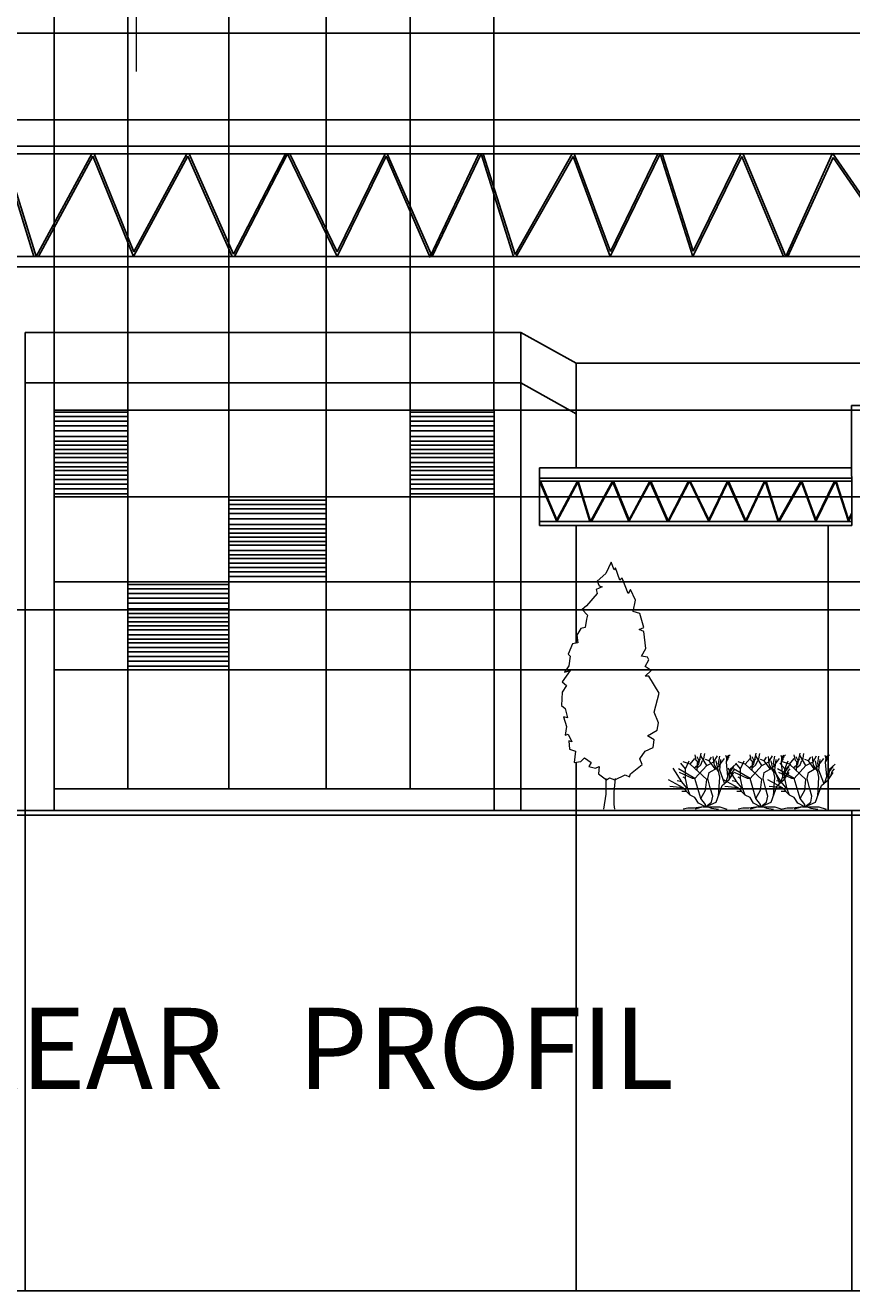
# Model space of a CAD drawing. Units: inches. Extents: x -32109 to 33221, y -19197 to 7608.
# Tile 3 of 25: x -12087 to -6953, y -19197 to -11338. Entities that reach past the tile are written whole.
import ezdxf

# ---------------------------------------------------------------- set-up
doc = ezdxf.new("R2010")
doc.units = ezdxf.units.IN
doc.header["$MEASUREMENT"] = 0
for name, color, linetype, lineweight in [('A-ANNO-DIMS', 2, 'Continuous', 18), ('A-ANNO-NOTE', 2, 'Continuous', 18), ('A-ANNO-TEXT', 7, 'Continuous', 25), ('A-ELEV', 7, 'Continuous', 25), ('L-PLNT', 3, 'Continuous', 13)]:
    doc.layers.add(name, color=color, linetype=linetype, lineweight=lineweight)
doc.styles.get("Standard").update_dxf_attribs({"font": 'arial.ttf'})
doc.dimstyles.get("Standard").update_dxf_attribs({"dimtxt": 0.18, "dimasz": 0.18, "dimexe": 0.18, "dimexo": 0.0625, "dimgap": 0.09, "dimtad": 0, "dimtih": 1, "dimtoh": 1, "dimdec": 4, "dimzin": 0, "dimdsep": 46, "dimtxsty": 'Standard', "dimcen": 0.09, "dimadec": 0, "dimazin": 0, "dimtfac": 1, "dimtdec": 4, "dimtofl": 0, "dimtmove": 0, "dimatfit": 3, "dimfxl": 1, "dimtolj": 1, "dimtzin": 0, "dimarcsym": 0})

# ---------------------------------------------------------------- blocks, each defined once
blk = doc.blocks.new('*U2')
blk.add_lwpolyline([(-2.754, 191.699), (-6.78, 182.851), (-13.682, 176.953), (-11.956, 173.266), (-9.656, 172.529), (-14.257, 170.317), (-13.682, 167.368), (-21.733, 157.783), (-25.184, 154.834), (-21.158, 150.41), (-21.733, 147.461), (-22.884, 140.825), (-26.334, 140.087), (-29.21, 134.926), (-28.635, 129.028), (-32.661, 128.291), (-36.111, 120.18), (-34.386, 118.706), (-35.536, 111.333), (-38.987, 106.171), (-34.386, 107.646), (-40.712, 98.798), (-37.261, 95.849), (-40.712, 90.688), (-41.287, 80.366), (-38.412, 78.154), (-36.686, 70.781), (-39.562, 71.518), (-37.261, 64.145), (-38.412, 57.509), (-36.111, 58.247), (-33.236, 52.348), (-35.536, 53.086), (-34.961, 46.45), (-30.36, 44.975), (-31.51, 36.128), (-26.334, 36.865), (-23.459, 39.814), (-18.283, 36.128), (-20.008, 33.178), (-14.832, 31.704), (-11.956, 33.178), (-12.531, 27.28), (-6.205, 22.856), (-3.905, 24.331), (0.121, 22.856), (8.173, 26.543), (11.624, 25.068), (12.199, 27.28), (21.4, 34.653), (19.675, 39.077), (23.701, 44.975), (30.027, 47.924), (30.602, 53.823), (25.426, 56.772), (32.903, 61.196), (34.053, 67.094), (30.602, 75.205), (34.628, 89.951), (26.576, 103.222), (23.701, 103.222), (28.302, 107.646), (23.701, 110.595), (26.576, 115.756), (25.426, 117.968), (20.825, 118.706), (24.276, 124.604), (22.551, 137.876), (19.1, 139.35), (22.551, 140.825), (19.675, 151.884), (14.499, 153.359), (16.224, 162.207), (12.199, 170.317), (10.473, 167.368), (5.872, 179.165), (4.147, 177.69), (0.696, 187.275), (-0.454, 185.8)], close=True)
for points in [[(-6.813, 23.669), (-6.813, 11.669), (-8.627, 0)], [(0.387, 23.669), (-0.576, 13.271), (-0.576, 3.686), (0, 0)]]:
    blk.add_lwpolyline(points)
blk = doc.blocks.new('*U3')
for p, q in [((-14.88, 18.24), (-12.96, 20.64)), ((-12.471, 19.775), (-12.898, 22.044)), ((-11.28, 19.619), (-12.104, 21.184)), ((-11.433, 18.289), (-10.457, 22.749)), ((-8.16, 17.76), (-10.56, 21.6)), ((-9.48, 19.775), (-8.992, 22.592)), ((-7.2, 19.68), (-6.24, 21.12)), ((-5.086, 17.741), (-5.513, 21.34)), ((-5.28, 19.2), (-3.84, 21.6)), ((-3.84, 16.8), (-0.96, 20.64)), ((-3.377, 18.602), (-2.888, 21.575)), ((-0.508, 21.888), (-0.081, 20.558)), ((-0.203, 19.149), (0.102, 21.34)), ((-0.02, 20.01), (0.896, 21.105)), ((0.041, 20.714), (1.384, 22.044)), ((0.102, 21.34), (0.835, 21.888)), ((-18.24, 11.04), (-21.755, 16.655)), ((-12.96, 12.48), (-19.68, 16.32)), ((-16.8, 16.32), (-18.72, 18.72)), ((-14.88, 18.24), (-17.76, 19.2)), ((-16.8, 16.32), (-15.36, 19.68)), ((-16.8, 12.48), (-16.8, 16.32)), ((-8.16, 12), (-14.88, 18.24)), ((-13.325, 16.724), (-11.433, 18.289)), ((-12.96, 12.48), (-8.16, 17.76)), ((-11.677, 19.071), (-12.471, 19.775)), ((-12.043, 15.628), (-11.921, 18.836)), ((-11.982, 16.802), (-10.579, 18.054)), ((-11.921, 18.836), (-10.64, 20.401)), ((-10.579, 18.054), (-9.846, 19.697)), ((-7.2, 19.68), (-8.64, 20.16)), ((-8.16, 17.76), (-5.28, 19.2)), ((-4.8, 16.32), (-7.2, 19.68)), ((-7.2, 14.88), (-3.84, 16.8)), ((-3.377, 15.315), (-5.086, 17.819)), ((-2.88, 12.96), (-4.32, 19.68)), ((-2.766, 16.802), (-3.377, 18.602)), ((-2.88, 15.84), (-2.4, 20.16)), ((-0.96, 10.56), (-2.88, 15.84)), ((0.346, 13.203), (-0.203, 19.149)), ((-0.142, 19.384), (0.59, 20.401)), ((0.346, 13.203), (1.323, 16.254)), ((1.323, 16.254), (3.642, 18.289)), ((1.44, 15.36), (2.88, 17.28)), ((2.4, 15.36), (3.36, 16.32)), ((-17.76, 8.64), (-23.663, 11.961)), ((-18.24, 11.04), (-20.16, 11.52)), ((-13.92, 12.48), (-19.2, 14.88)), ((-15.84, 8.16), (-18.24, 11.04)), ((-16.8, 12.48), (-17.76, 12.96)), ((-15.84, 8.16), (-16.8, 12.48)), ((-12.96, 12.48), (-13.92, 12.48)), ((-10.56, 4.32), (-12.96, 12.48)), ((-8.64, 7.68), (-8.16, 12)), ((-7.68, 12.48), (-7.2, 14.88)), ((-6.72, 8.64), (-7.68, 12.48)), ((-3.36, 5.28), (-2.88, 12.96)), ((-1.92, 9.6), (0.96, 12)), ((-0.48, 10.8), (0.346, 13.203)), ((0.96, 12), (1.44, 15.36)), ((0.96, 12), (2.88, 14.88)), ((1.92, 13.44), (2.4, 15.36)), ((-17.76, 8.64), (-23.128, 9.222)), ((-16.32, 7.2), (-18.24, 7.2)), ((-14.88, 5.76), (-17.76, 8.64)), ((-14.88, 5.76), (-15.84, 8.16)), ((-12.96, 4.8), (-14.88, 5.76)), ((-10.56, 4.32), (-8.64, 7.68)), ((-5.76, 5.28), (-6.72, 8.64)), ((-6.24, 2.88), (-5.76, 5.28)), ((-4.32, 2.88), (-1.92, 9.6)), ((-15.84, 0.48), (-17.76, 0)), ((-13.44, 0.48), (-15.84, 0.48)), ((-9.6, 0.96), (-13.44, 0.48)), ((-11.52, 2.4), (-12.96, 4.8)), ((-9.6, 0.96), (-12.96, 0)), ((-8.64, 0.96), (-11.52, 2.4)), ((-8.64, 1.92), (-10.56, 4.32)), ((-9.6, 0.96), (-7.68, 0.96)), ((-8.64, 0.96), (-4.32, 2.88)), ((-8.64, 0.96), (-6.24, 2.88)), ((-8.64, 0.96), (-8.64, 1.92)), ((-8.64, 0.96), (-2.88, 0.96)), ((-7.68, 0.96), (-6.24, 0.48)), ((-6.24, 0.48), (-3.36, 0)), ((-2.88, 0.96), (0, 0))]:
    blk.add_line(p, q)
blk = doc.blocks.new('*D13')
at = {"layer": 'A-ANNO-DIMS', "color": 0, "lineweight": -2, "transparency": 16777216}
for p, q in [((-21916.3, -16214.9), (-21916.3, -19197.3)), ((5067.2, -16244.2), (5067.2, -19197.3)), ((-21916.1, -19197.2), (-8425, -19197.2)), ((5067, -19197.2), (-8424.2, -19197.2))]:
    blk.add_line(p, q, dxfattribs=at)
at = {"layer": 'A-ANNO-DIMS', "color": 0, "transparency": 16777216}
for points in [[(-21916.1, -19197.1), (-21916.1, -19197.2), (-21916.3, -19197.2)], [(5067, -19197.1), (5067, -19197.2), (5067.2, -19197.2)]]:
    blk.add_solid(points, dxfattribs=at)
at = {"layer": 'Defpoints', "color": 0, "transparency": 16777216}
for p in [(-21916.3, -16214.8), (5067.2, -16244.1), (5067.2, -19197.2)]:
    blk.add_point(p, dxfattribs=at)
at = {"layer": 'A-ANNO-DIMS', "color": 0, "transparency": 16777216, "insert": (-8424.6, -19197.2), "char_height": 0.18, "attachment_point": 5}
blk.add_mtext('\\A1;26983', dxfattribs=at)
blk = doc.blocks.new('*D14')
at = {"layer": 'A-ANNO-DIMS', "color": 0, "lineweight": -2, "transparency": 16777216}
for p, q in [((-18893.9, -10978.7), (-32108.4, -10978.7)), ((-32108.2, -10978.9), (-32108.2, -13611.2)), ((-32108.2, -16243.9), (-32108.2, -13611.6)), ((5067.1, -16244.1), (-32108.4, -16244.1))]:
    blk.add_line(p, q, dxfattribs=at)
at = {"layer": 'A-ANNO-DIMS', "color": 0, "transparency": 16777216}
for points in [[(-32108.2, -10978.9), (-32108.2, -10978.9), (-32108.2, -10978.7)], [(-32108.2, -16243.9), (-32108.2, -16243.9), (-32108.2, -16244.1)]]:
    blk.add_solid(points, dxfattribs=at)
at = {"layer": 'Defpoints', "color": 0, "transparency": 16777216}
for p in [(-18893.8, -10978.7), (-32108.2, -16244.1), (5067.2, -16244.1)]:
    blk.add_point(p, dxfattribs=at)
at = {"layer": 'A-ANNO-DIMS', "color": 0, "transparency": 16777216, "insert": (-32108.2, -13611.4), "char_height": 0.18, "attachment_point": 5}
blk.add_mtext('\\A1;5265', dxfattribs=at)
blk = doc.blocks.new('*D15')
at = {"layer": 'A-ANNO-DIMS', "color": 0, "lineweight": -2, "transparency": 16777216}
for p, q in [((-8664.1, -16214.9), (-8664.1, -19197.3)), ((-6952.8, -16214.9), (-6952.8, -19197.3)), ((-8664, -19197.2), (-7808.9, -19197.2)), ((-6953, -19197.2), (-7808, -19197.2))]:
    blk.add_line(p, q, dxfattribs=at)
at = {"layer": 'A-ANNO-DIMS', "color": 0, "transparency": 16777216}
for points in [[(-8664, -19197.1), (-8664, -19197.2), (-8664.1, -19197.2)], [(-6953, -19197.1), (-6953, -19197.2), (-6952.8, -19197.2)]]:
    blk.add_solid(points, dxfattribs=at)
at = {"layer": 'Defpoints', "color": 0, "transparency": 16777216}
for p in [(-8664.1, -16214.8), (-6952.8, -16214.8), (-6952.8, -19197.2)]:
    blk.add_point(p, dxfattribs=at)
at = {"layer": 'A-ANNO-DIMS', "color": 0, "transparency": 16777216, "insert": (-7808.5, -19197.2), "char_height": 0.18, "attachment_point": 5}
blk.add_mtext('\\A1;1711.4', dxfattribs=at)
blk = doc.blocks.new('*D23')
at = {"layer": 'A-ANNO-DIMS', "color": 0, "lineweight": -2, "transparency": 16777216}
for p, q in [((-4093.7, -14968.1), (-32108.4, -14968.1)), ((-32108.2, -14968.3), (-32108.2, -15591.3)), ((-32108.2, -16214.6), (-32108.2, -15591.6)), ((-4279, -16214.8), (-32108.4, -16214.8))]:
    blk.add_line(p, q, dxfattribs=at)
at = {"layer": 'A-ANNO-DIMS', "color": 0, "transparency": 16777216}
for points in [[(-32108.2, -14968.3), (-32108.2, -14968.3), (-32108.2, -14968.1)], [(-32108.2, -16214.6), (-32108.2, -16214.6), (-32108.2, -16214.8)]]:
    blk.add_solid(points, dxfattribs=at)
at = {"layer": 'Defpoints', "color": 0, "transparency": 16777216}
for p in [(-32108.2, -14968.1), (-4093.7, -14968.1), (-4279, -16214.8)]:
    blk.add_point(p, dxfattribs=at)
at = {"layer": 'A-ANNO-DIMS', "color": 0, "transparency": 16777216, "insert": (-32108.2, -15591.4), "char_height": 0.18, "attachment_point": 5}
blk.add_mtext('\\A1;1246.7', dxfattribs=at)
blk = doc.blocks.new('*D83')
at = {"layer": 'A-ANNO-DIMS', "color": 0, "lineweight": -2, "transparency": 16777216}
for p, q in [((-12087.2, -16214.9), (-12087.2, -19197.3)), ((-8664.1, -16214.9), (-8664.1, -19197.3)), ((-12087, -19197.2), (-10376, -19197.2)), ((-8664.3, -19197.2), (-10375.3, -19197.2))]:
    blk.add_line(p, q, dxfattribs=at)
at = {"layer": 'A-ANNO-DIMS', "color": 0, "transparency": 16777216}
for points in [[(-12087, -19197.1), (-12087, -19197.2), (-12087.2, -19197.2)], [(-8664.3, -19197.1), (-8664.3, -19197.2), (-8664.1, -19197.2)]]:
    blk.add_solid(points, dxfattribs=at)
at = {"layer": 'Defpoints', "color": 0, "transparency": 16777216}
for p in [(-12087.2, -16214.8), (-8664.1, -16214.8), (-8664.1, -19197.2)]:
    blk.add_point(p, dxfattribs=at)
at = {"layer": 'A-ANNO-DIMS', "color": 0, "transparency": 16777216, "insert": (-10375.7, -19197.2), "char_height": 0.18, "attachment_point": 5}
blk.add_mtext('\\A1;3423', dxfattribs=at)
blk = doc.blocks.new('*D88')
at = {"layer": 'A-ANNO-DIMS', "color": 0, "lineweight": -2, "transparency": 16777216}
for p, q in [((-6450, -11924), (-32108.4, -11924)), ((-32108.2, -11924.1), (-32108.2, -12380.7)), ((-32108.2, -12837.6), (-32108.2, -12381)), ((-6450, -12837.7), (-32108.4, -12837.7))]:
    blk.add_line(p, q, dxfattribs=at)
at = {"layer": 'A-ANNO-DIMS', "color": 0, "transparency": 16777216}
for points in [[(-32108.2, -11924.1), (-32108.2, -11924.1), (-32108.2, -11924)], [(-32108.2, -12837.6), (-32108.2, -12837.6), (-32108.2, -12837.7)]]:
    blk.add_solid(points, dxfattribs=at)
at = {"layer": 'Defpoints', "color": 0, "transparency": 16777216}
for p in [(-6450, -11924), (-32108.2, -12837.7), (-6450, -12837.7)]:
    blk.add_point(p, dxfattribs=at)
at = {"layer": 'A-ANNO-DIMS', "color": 0, "transparency": 16777216, "insert": (-32108.2, -12380.9), "char_height": 0.18, "attachment_point": 5}
blk.add_mtext('\\A1;913.8', dxfattribs=at)
blk = doc.blocks.new('*D92')
at = {"layer": 'A-ANNO-DIMS', "color": 0, "lineweight": -2, "transparency": 16777216}
for p, q in [((-8664.1, -13437.2), (9252.7, -13437.2)), ((9252.5, -13437.4), (9252.5, -14825.8)), ((9252.5, -16214.6), (9252.5, -14826.2)), ((-8664.1, -16214.8), (9252.7, -16214.8))]:
    blk.add_line(p, q, dxfattribs=at)
at = {"layer": 'A-ANNO-DIMS', "color": 0, "transparency": 16777216}
for points in [[(9252.5, -13437.4), (9252.5, -13437.4), (9252.5, -13437.2)], [(9252.5, -16214.6), (9252.5, -16214.6), (9252.5, -16214.8)]]:
    blk.add_solid(points, dxfattribs=at)
at = {"layer": 'Defpoints', "color": 0, "transparency": 16777216}
for p in [(-8664.1, -13437.2), (-8664.1, -16214.8), (9252.5, -16214.8)]:
    blk.add_point(p, dxfattribs=at)
at = {"layer": 'A-ANNO-DIMS', "color": 0, "transparency": 16777216, "insert": (9252.5, -14826), "char_height": 0.18, "attachment_point": 5}
blk.add_mtext('\\A1;2777.6', dxfattribs=at)
blk = doc.blocks.new('*D94')
at = {"layer": 'A-ANNO-DIMS', "color": 0, "lineweight": -2, "transparency": 16777216}
for p, q in [((-11907.7, -13729), (-11907.7, -7335)), ((-11907.5, -7335.2), (-11679.5, -7335.2)), ((-11450.7, -7335.2), (-11678.7, -7335.2)), ((-11450.5, -13729), (-11450.5, -7335))]:
    blk.add_line(p, q, dxfattribs=at)
at = {"layer": 'A-ANNO-DIMS', "color": 0, "transparency": 16777216}
for points in [[(-11907.5, -7335.1), (-11907.5, -7335.2), (-11907.7, -7335.2)], [(-11450.7, -7335.1), (-11450.7, -7335.2), (-11450.5, -7335.2)]]:
    blk.add_solid(points, dxfattribs=at)
at = {"layer": 'Defpoints', "color": 0, "transparency": 16777216}
for p in [(-11450.5, -7335.2), (-11907.7, -13729), (-11450.5, -13729)]:
    blk.add_point(p, dxfattribs=at)
at = {"layer": 'A-ANNO-DIMS', "color": 0, "transparency": 16777216, "insert": (-11679.1, -7335.2), "char_height": 0.18, "attachment_point": 5}
blk.add_mtext('\\A1;457.2', dxfattribs=at)
blk = doc.blocks.new('*D95')
at = {"layer": 'A-ANNO-DIMS', "color": 0, "lineweight": -2, "transparency": 16777216}
for p, q in [((-11450.5, -13729), (-11450.5, -7335)), ((-11450.3, -7335.2), (-11137.2, -7335.2)), ((-10823.3, -7335.2), (-11136.4, -7335.2)), ((-10823.2, -13729), (-10823.2, -7335))]:
    blk.add_line(p, q, dxfattribs=at)
at = {"layer": 'A-ANNO-DIMS', "color": 0, "transparency": 16777216}
for points in [[(-11450.3, -7335.1), (-11450.3, -7335.2), (-11450.5, -7335.2)], [(-10823.3, -7335.1), (-10823.3, -7335.2), (-10823.2, -7335.2)]]:
    blk.add_solid(points, dxfattribs=at)
at = {"layer": 'Defpoints', "color": 0, "transparency": 16777216}
for p in [(-10823.2, -7335.2), (-11450.5, -13729), (-10823.2, -13729)]:
    blk.add_point(p, dxfattribs=at)
at = {"layer": 'A-ANNO-DIMS', "color": 0, "transparency": 16777216, "insert": (-11136.8, -7335.2), "char_height": 0.18, "attachment_point": 5}
blk.add_mtext('\\A1;627.3', dxfattribs=at)
blk = doc.blocks.new('*D96')
at = {"layer": 'A-ANNO-DIMS', "color": 0, "lineweight": -2, "transparency": 16777216}
for p, q in [((-10823.2, -13729), (-10823.2, -7335)), ((-10823, -7335.2), (-10520.4, -7335.2)), ((-10217.3, -7335.2), (-10519.9, -7335.2)), ((-10217.1, -13729), (-10217.1, -7335))]:
    blk.add_line(p, q, dxfattribs=at)
at = {"layer": 'A-ANNO-DIMS', "color": 0, "transparency": 16777216}
for points in [[(-10823, -7335.1), (-10823, -7335.2), (-10823.2, -7335.2)], [(-10217.3, -7335.1), (-10217.3, -7335.2), (-10217.1, -7335.2)]]:
    blk.add_solid(points, dxfattribs=at)
at = {"layer": 'Defpoints', "color": 0, "transparency": 16777216}
for p in [(-10217.1, -7335.2), (-10823.2, -13729), (-10217.1, -13729)]:
    blk.add_point(p, dxfattribs=at)
at = {"layer": 'A-ANNO-DIMS', "color": 0, "transparency": 16777216, "insert": (-10520.1, -7335.2), "char_height": 0.18, "attachment_point": 5}
blk.add_mtext('\\A1;606', dxfattribs=at)
blk = doc.blocks.new('*D97')
at = {"layer": 'A-ANNO-DIMS', "color": 0, "lineweight": -2, "transparency": 16777216}
for p, q in [((-10217.1, -13729), (-10217.1, -7335)), ((-10216.9, -7335.2), (-9956.9, -7335.2)), ((-9696.3, -7335.2), (-9956.4, -7335.2)), ((-9696.1, -13729), (-9696.1, -7335))]:
    blk.add_line(p, q, dxfattribs=at)
at = {"layer": 'A-ANNO-DIMS', "color": 0, "transparency": 16777216}
for points in [[(-10216.9, -7335.1), (-10216.9, -7335.2), (-10217.1, -7335.2)], [(-9696.3, -7335.1), (-9696.3, -7335.2), (-9696.1, -7335.2)]]:
    blk.add_solid(points, dxfattribs=at)
at = {"layer": 'Defpoints', "color": 0, "transparency": 16777216}
for p in [(-9696.1, -7335.2), (-10217.1, -13729), (-9696.1, -13729)]:
    blk.add_point(p, dxfattribs=at)
at = {"layer": 'A-ANNO-DIMS', "color": 0, "transparency": 16777216, "insert": (-9956.6, -7335.2), "char_height": 0.18, "attachment_point": 5}
blk.add_mtext('\\A1;521', dxfattribs=at)
blk = doc.blocks.new('*D98')
at = {"layer": 'A-ANNO-DIMS', "color": 0, "lineweight": -2, "transparency": 16777216}
for p, q in [((-9696.1, -13729), (-9696.1, -7335)), ((-9696, -7335.2), (-9435.9, -7335.2)), ((-9175.3, -7335.2), (-9435.4, -7335.2)), ((-9175.2, -13729), (-9175.2, -7335))]:
    blk.add_line(p, q, dxfattribs=at)
at = {"layer": 'A-ANNO-DIMS', "color": 0, "transparency": 16777216}
for points in [[(-9696, -7335.1), (-9696, -7335.2), (-9696.1, -7335.2)], [(-9175.3, -7335.1), (-9175.3, -7335.2), (-9175.2, -7335.2)]]:
    blk.add_solid(points, dxfattribs=at)
at = {"layer": 'Defpoints', "color": 0, "transparency": 16777216}
for p in [(-9175.2, -7335.2), (-9696.1, -13729), (-9175.2, -13729)]:
    blk.add_point(p, dxfattribs=at)
at = {"layer": 'A-ANNO-DIMS', "color": 0, "transparency": 16777216, "insert": (-9435.6, -7335.2), "char_height": 0.18, "attachment_point": 5}
blk.add_mtext('\\A1;521', dxfattribs=at)
blk = doc.blocks.new('*D99')
at = {"layer": 'A-ANNO-DIMS', "color": 0, "lineweight": -2, "transparency": 16777216}
for p, q in [((-9175.1, -13729), (9252.7, -13729)), ((9252.5, -13729.2), (9252.5, -13997.5)), ((9252.5, -14266.2), (9252.5, -13997.9)), ((-9175.1, -14266.4), (9252.7, -14266.4))]:
    blk.add_line(p, q, dxfattribs=at)
at = {"layer": 'A-ANNO-DIMS', "color": 0, "transparency": 16777216}
for points in [[(9252.5, -13729.2), (9252.5, -13729.2), (9252.5, -13729)], [(9252.5, -14266.2), (9252.5, -14266.2), (9252.5, -14266.4)]]:
    blk.add_solid(points, dxfattribs=at)
at = {"layer": 'Defpoints', "color": 0, "transparency": 16777216}
for p in [(-9175.2, -13729), (-9175.2, -14266.4), (9252.5, -14266.4)]:
    blk.add_point(p, dxfattribs=at)
at = {"layer": 'A-ANNO-DIMS', "color": 0, "transparency": 16777216, "insert": (9252.5, -13997.7), "char_height": 0.18, "attachment_point": 5}
blk.add_mtext('\\A1;537.4', dxfattribs=at)
blk = doc.blocks.new('*D100')
at = {"layer": 'A-ANNO-DIMS', "color": 0, "lineweight": -2, "transparency": 16777216}
for p, q in [((-9175.1, -14266.4), (9252.7, -14266.4)), ((9252.5, -14266.6), (9252.5, -14530.6)), ((9252.5, -14794.9), (9252.5, -14530.9)), ((-9175.1, -14795.1), (9252.7, -14795.1))]:
    blk.add_line(p, q, dxfattribs=at)
at = {"layer": 'A-ANNO-DIMS', "color": 0, "transparency": 16777216}
for points in [[(9252.5, -14266.6), (9252.5, -14266.6), (9252.5, -14266.4)], [(9252.5, -14794.9), (9252.5, -14794.9), (9252.5, -14795.1)]]:
    blk.add_solid(points, dxfattribs=at)
at = {"layer": 'Defpoints', "color": 0, "transparency": 16777216}
for p in [(-9175.2, -14266.4), (-9175.2, -14795.1), (9252.5, -14795.1)]:
    blk.add_point(p, dxfattribs=at)
at = {"layer": 'A-ANNO-DIMS', "color": 0, "transparency": 16777216, "insert": (9252.5, -14530.7), "char_height": 0.18, "attachment_point": 5}
blk.add_mtext('\\A1;528.7', dxfattribs=at)
blk = doc.blocks.new('*D101')
at = {"layer": 'A-ANNO-DIMS', "color": 0, "lineweight": -2, "transparency": 16777216}
for p, q in [((-9175.1, -14795.1), (9252.7, -14795.1)), ((9252.5, -14795.3), (9252.5, -15068.4)), ((9252.5, -15341.8), (9252.5, -15068.7)), ((-9175.1, -15342), (9252.7, -15342))]:
    blk.add_line(p, q, dxfattribs=at)
at = {"layer": 'A-ANNO-DIMS', "color": 0, "transparency": 16777216}
for points in [[(9252.5, -14795.3), (9252.5, -14795.3), (9252.5, -14795.1)], [(9252.5, -15341.8), (9252.5, -15341.8), (9252.5, -15342)]]:
    blk.add_solid(points, dxfattribs=at)
at = {"layer": 'Defpoints', "color": 0, "transparency": 16777216}
for p in [(-9175.2, -14795.1), (-9175.2, -15342), (9252.5, -15342)]:
    blk.add_point(p, dxfattribs=at)
at = {"layer": 'A-ANNO-DIMS', "color": 0, "transparency": 16777216, "insert": (9252.5, -15068.6), "char_height": 0.18, "attachment_point": 5}
blk.add_mtext('\\A1;546.9', dxfattribs=at)
blk = doc.blocks.new('*D102')
at = {"layer": 'A-ANNO-DIMS', "color": 0, "lineweight": -2, "transparency": 16777216}
for p, q in [((-9175.1, -15342), (9252.7, -15342)), ((9252.5, -15342.2), (9252.5, -15710.5)), ((9252.5, -16079.1), (9252.5, -15710.8)), ((-9175.1, -16079.3), (9252.7, -16079.3))]:
    blk.add_line(p, q, dxfattribs=at)
at = {"layer": 'A-ANNO-DIMS', "color": 0, "transparency": 16777216}
for points in [[(9252.5, -15342.2), (9252.5, -15342.2), (9252.5, -15342)], [(9252.5, -16079.1), (9252.5, -16079.1), (9252.5, -16079.3)]]:
    blk.add_solid(points, dxfattribs=at)
at = {"layer": 'Defpoints', "color": 0, "transparency": 16777216}
for p in [(-9175.2, -15342), (-9175.2, -16079.3), (9252.5, -16079.3)]:
    blk.add_point(p, dxfattribs=at)
at = {"layer": 'A-ANNO-DIMS', "color": 0, "transparency": 16777216, "insert": (9252.5, -15710.6), "char_height": 0.18, "attachment_point": 5}
blk.add_mtext('\\A1;737.3', dxfattribs=at)
blk = doc.blocks.new('*D111')
at = {"layer": 'A-ANNO-DIMS', "color": 0, "lineweight": -2, "transparency": 16777216}
for p, q in [((-6954.6, -13699.5), (9252.7, -13699.5)), ((9252.5, -13699.6), (9252.5, -14957)), ((9252.5, -16214.6), (9252.5, -14957.3)), ((-6952.7, -16214.8), (9252.7, -16214.8))]:
    blk.add_line(p, q, dxfattribs=at)
at = {"layer": 'A-ANNO-DIMS', "color": 0, "transparency": 16777216}
for points in [[(9252.5, -13699.6), (9252.5, -13699.6), (9252.5, -13699.5)], [(9252.5, -16214.6), (9252.5, -16214.6), (9252.5, -16214.8)]]:
    blk.add_solid(points, dxfattribs=at)
at = {"layer": 'Defpoints', "color": 0, "transparency": 16777216}
for p in [(-6954.6, -13699.5), (-6952.8, -16214.8), (9252.5, -16214.8)]:
    blk.add_point(p, dxfattribs=at)
at = {"layer": 'A-ANNO-DIMS', "color": 0, "transparency": 16777216, "insert": (9252.5, -14957.1), "char_height": 0.18, "attachment_point": 5}
blk.add_mtext('\\A1;2515.4', dxfattribs=at)
blk = doc.blocks.new('*D159')
at = {"layer": 'A-ANNO-DIMS', "color": 0, "lineweight": -2, "transparency": 16777216}
for p, q in [((-6094.7, -11386.3), (-32108.4, -11386.3)), ((-32108.2, -11386.4), (-32108.2, -13800.4)), ((-32108.2, -16214.6), (-32108.2, -13800.7)), ((-6952.8, -16214.8), (-32108.4, -16214.8))]:
    blk.add_line(p, q, dxfattribs=at)
at = {"layer": 'A-ANNO-DIMS', "color": 0, "transparency": 16777216}
for points in [[(-32108.2, -11386.4), (-32108.2, -11386.4), (-32108.2, -11386.3)], [(-32108.2, -16214.6), (-32108.2, -16214.6), (-32108.2, -16214.8)]]:
    blk.add_solid(points, dxfattribs=at)
at = {"layer": 'Defpoints', "color": 0, "transparency": 16777216}
for p in [(-6094.7, -11386.3), (-32108.2, -16214.8), (-6952.8, -16214.8)]:
    blk.add_point(p, dxfattribs=at)
at = {"layer": 'A-ANNO-DIMS', "color": 0, "transparency": 16777216, "insert": (-32108.2, -13800.5), "char_height": 0.18, "attachment_point": 5}
blk.add_mtext('\\A1;4828.6', dxfattribs=at)

msp = doc.modelspace()

# ---------------------------------------------------------------- linework, layer by layer
at = {"layer": 'A-ANNO-NOTE'}
msp.add_line((-11395.932, -11625.267), (-11395.932, -9225.16), dxfattribs=at)
at = {"layer": 'A-ELEV'}
for p, q in [((-6449.955, -11923.964), (-13434.383, -11923.964)), ((-13434.383, -12088.725), (-6449.955, -12088.725)), ((-6449.955, -12135.164), (-13434.383, -12135.164)), ((-12033.808, -12773.917), (-12224.259, -12151.939)), ((-12020.326, -12774.298), (-12215.76, -12136.047)), ((-11673.548, -12136.139), (-12020.326, -12774.298)), ((-11667.326, -12151.455), (-12005.574, -12773.917)), ((-11414.231, -12774.408), (-11667.326, -12151.455)), ((-11412.588, -12744.499), (-11660.15, -12135.164)), ((-11076.952, -12150.578), (-11414.231, -12774.408)), ((-11083.147, -12135.164), (-11412.588, -12744.499)), ((-10802.158, -12773.917), (-11076.952, -12150.578)), ((-10794.601, -12759.378), (-11069.259, -12136.348)), ((-10471.397, -12135.164), (-10794.601, -12759.378)), ((-10457.568, -12136.249), (-10787.983, -12774.39)), ((-10148.844, -12774.323), (-10457.568, -12136.249)), ((-10148.814, -12745.042), (-10443.896, -12135.164)), ((-9845.785, -12151.2), (-10148.844, -12774.323)), ((-9852.197, -12135.164), (-10148.814, -12745.042)), ((-9570.82, -12779.373), (-9845.785, -12151.2)), ((-9559.112, -12774.249), (-9838.443, -12136.104)), ((-9269.526, -12135.164), (-9570.655, -12768.763)), ((-9255.782, -12136.019), (-9559.112, -12774.249)), ((-9053.761, -12773.917), (-9255.782, -12136.019)), ((-9044.471, -12760.923), (-9242.647, -12135.164)), ((-8690.019, -12136.482), (-9044.471, -12760.923)), ((-8684.219, -12152.151), (-9037.152, -12773.917)), ((-8453.963, -12774.128), (-8684.219, -12152.151)), ((-8452.368, -12741.626), (-8676.88, -12135.164)), ((-8143.814, -12136.351), (-8453.963, -12774.128)), ((-8157.448, -12135.164), (-8452.368, -12741.626)), ((-7939.481, -12774.128), (-8143.814, -12136.351)), ((-7936.987, -12740.027), (-8130.775, -12135.164)), ((-7634.998, -12153.442), (-7939.481, -12774.128)), ((-7638.981, -12132.545), (-7936.987, -12740.027)), ((-7376.899, -12773.917), (-7634.998, -12153.442)), ((-7362.969, -12774.128), (-7627.508, -12138.174)), ((-7071.065, -12132.707), (-7362.969, -12774.128)), ((-7068.778, -12158.535), (-7348.832, -12773.917)), ((-6628.917, -12773.917), (-7071.065, -12132.707)), ((-6644.441, -12773.917), (-7068.778, -12158.535)), ((-13434.383, -12773.917), (-6449.955, -12773.917)), ((-10787.983, -12774.39), (-10788.191, -12773.917)), ((-6449.955, -12837.747), (-13434.383, -12837.747)), ((-12087.226, -12837.489), (-9386.71, -12837.747)), ((-9070.682, -12837.747), (-11681.584, -12837.747)), ((-12087.226, -13436.327), (-12087.226, -13244.79)), ((-12087.226, -13244.79), (-9009.085, -13244.79)), ((-9009.085, -13244.79), (-8664.143, -13437.203)), ((-9009.085, -13244.79), (-9009.085, -13557.609)), ((-12087.226, -14445.256), (-12087.226, -13436.327)), ((-8664.143, -13750.022), (-8664.143, -13437.203)), ((-9009.085, -13557.609), (-12087.226, -13557.609)), ((-9009.085, -13557.609), (-9009.085, -14445.256)), ((-9009.085, -13557.609), (-8664.143, -13750.022)), ((-11907.664, -16214.811), (-11907.664, -13729.028)), ((-11907.664, -13729.028), (-9175.157, -13729.028)), ((-11907.664, -13741.003), (-11450.474, -13741.003)), ((-11450.474, -16079.3), (-11450.474, -13729.028)), ((-10823.167, -16079.3), (-10823.167, -13729.028)), ((-10217.124, -16079.3), (-10217.124, -13729.028)), ((-9699.007, -13741.003), (-9175.157, -13741.003)), ((-9696.14, -16079.3), (-9696.14, -13729.028)), ((-9175.157, -13729.028), (-9175.157, -16214.811)), ((-8664.143, -14086.672), (-8664.143, -13750.022)), ((-6954.623, -13834.091), (-6954.623, -13699.459)), ((-6954.623, -13699.459), (-6943.296, -13699.459)), ((-11907.664, -13768.233), (-11450.474, -13768.233)), ((-11907.664, -13796.415), (-11450.474, -13796.415)), ((-11907.664, -13824.813), (-11450.474, -13824.813)), ((-9699.007, -13768.233), (-9175.157, -13768.233)), ((-9699.007, -13796.415), (-9175.157, -13796.415)), ((-9699.007, -13824.813), (-9175.157, -13824.813)), ((-11907.664, -13857.368), (-11450.474, -13857.368)), ((-11907.664, -13892), (-11450.474, -13892)), ((-9699.007, -13857.368), (-9175.157, -13857.368)), ((-9699.007, -13892), (-9175.157, -13892)), ((-6954.623, -13834.091), (-6952.774, -14445.256)), ((-11907.664, -13919.943), (-11450.474, -13919.943)), ((-11907.664, -13946.263), (-11450.474, -13946.263)), ((-11907.664, -13971.892), (-11450.474, -13971.892)), ((-9699.007, -13919.943), (-9175.157, -13919.943)), ((-9699.007, -13946.263), (-9175.157, -13946.263)), ((-9699.007, -13971.892), (-9175.157, -13971.892)), ((-11907.664, -13997.52), (-11450.474, -13997.52)), ((-11907.664, -14021.762), (-11450.474, -14021.762)), ((-11907.664, -14053.653), (-11450.474, -14053.653)), ((-9699.007, -13997.52), (-9175.157, -13997.52)), ((-9699.007, -14021.762), (-9175.157, -14021.762)), ((-9699.007, -14053.653), (-9175.157, -14053.653)), ((-11907.664, -14080.587), (-11450.474, -14080.587)), ((-11907.664, -14103.611), (-11450.474, -14103.611)), ((-11907.664, -14132.215), (-11450.474, -14132.215)), ((-9699.007, -14080.587), (-9175.157, -14080.587)), ((-9699.007, -14103.611), (-9175.157, -14103.611)), ((-9699.007, -14132.215), (-9175.157, -14132.215)), ((-6953.859, -14086.672), (-8891.72, -14086.672)), ((-8891.72, -14086.672), (-8891.72, -14151.327)), ((-11907.664, -14159.446), (-11450.474, -14159.446)), ((-11907.664, -14187.627), (-11450.474, -14187.627)), ((-11907.664, -14216.026), (-11450.474, -14216.026)), ((-9699.007, -14159.446), (-9175.157, -14159.446)), ((-9699.007, -14187.627), (-9175.157, -14187.627)), ((-9699.007, -14216.026), (-9175.157, -14216.026)), ((-8891.72, -14151.327), (-6953.663, -14151.327)), ((-8891.72, -14169.551), (-8891.72, -14151.327)), ((-8785.46, -14420.382), (-8891.72, -14169.464)), ((-6953.608, -14169.551), (-8891.72, -14169.551)), ((-8891.72, -14169.551), (-8891.72, -14420.208)), ((-8784.934, -14408.765), (-8886.237, -14169.551)), ((-8654.831, -14176.133), (-8785.46, -14420.382)), ((-8656.997, -14169.551), (-8784.934, -14408.765)), ((-8580.094, -14420.208), (-8654.831, -14176.133)), ((-8574.804, -14420.357), (-8651.495, -14169.897)), ((-8438.722, -14169.933), (-8574.804, -14420.357)), ((-8436.281, -14175.943), (-8569.015, -14420.208)), ((-8336.962, -14420.4), (-8436.281, -14175.943)), ((-8336.317, -14408.664), (-8433.465, -14169.551)), ((-8204.608, -14175.599), (-8336.962, -14420.4)), ((-8207.039, -14169.551), (-8336.317, -14408.664)), ((-8096.774, -14420.208), (-8204.608, -14175.599)), ((-8093.809, -14414.502), (-8201.589, -14170.015)), ((-7966.978, -14169.551), (-8093.809, -14414.502)), ((-7961.551, -14169.976), (-8091.212, -14420.394)), ((-7840.403, -14420.367), (-7961.551, -14169.976)), ((-7840.391, -14408.877), (-7956.186, -14169.551)), ((-7721.477, -14175.843), (-7840.403, -14420.367)), ((-7723.994, -14169.551), (-7840.391, -14408.877)), ((-7613.576, -14422.349), (-7721.477, -14175.843)), ((-7608.982, -14420.338), (-7718.596, -14169.919)), ((-7495.344, -14169.551), (-7613.512, -14418.185)), ((-7489.95, -14169.886), (-7608.982, -14420.338)), ((-7410.674, -14420.208), (-7489.95, -14169.886)), ((-7407.029, -14415.109), (-7484.796, -14169.551)), ((-7267.936, -14170.068), (-7407.029, -14415.109)), ((-7265.659, -14176.217), (-7404.156, -14420.208)), ((-7175.303, -14420.291), (-7265.659, -14176.217)), ((-7174.677, -14407.536), (-7262.78, -14169.551)), ((-7053.596, -14170.016), (-7175.303, -14420.291)), ((-7058.946, -14169.551), (-7174.677, -14407.536)), ((-6973.412, -14420.291), (-7053.596, -14170.016)), ((-6972.433, -14406.909), (-7048.479, -14169.551)), ((-11907.664, -14248.581), (-11450.474, -14248.581)), ((-11907.664, -14266.38), (-9175.157, -14266.38)), ((-10823.167, -14286.356), (-10217.124, -14286.356)), ((-9699.007, -14248.581), (-9175.157, -14248.581)), ((-10823.167, -14313.587), (-10217.124, -14313.587)), ((-10823.167, -14341.768), (-10217.124, -14341.768)), ((-10823.167, -14370.167), (-10217.124, -14370.167)), ((-6952.975, -14378.631), (-6973.412, -14420.291)), ((-6953.01, -14367.314), (-6972.433, -14406.909)), ((-12087.226, -14445.256), (-12087.226, -16214.811)), ((-10823.167, -14402.721), (-10217.124, -14402.721)), ((-10823.167, -14437.354), (-10217.124, -14437.354)), ((-9009.085, -14445.256), (-9009.085, -16214.811)), ((-8891.72, -14420.208), (-6952.85, -14420.208)), ((-8891.72, -14445.256), (-8891.72, -14420.208)), ((-6952.774, -14445.256), (-8891.72, -14445.256)), ((-8664.143, -14445.256), (-8664.143, -15175.201)), ((-8091.212, -14420.394), (-8091.294, -14420.208)), ((-7098.526, -14445.256), (-7098.526, -16214.811)), ((-10823.167, -14465.296), (-10217.124, -14465.296)), ((-10823.167, -14491.617), (-10217.124, -14491.617)), ((-10823.167, -14517.245), (-10217.124, -14517.245)), ((-10823.167, -14542.873), (-10217.124, -14542.873)), ((-10823.167, -14567.116), (-10217.124, -14567.116)), ((-10823.167, -14599.007), (-10217.124, -14599.007)), ((-10823.167, -14625.941), (-10217.124, -14625.941)), ((-10823.167, -14648.965), (-10217.124, -14648.965)), ((-10823.167, -14677.569), (-10217.124, -14677.569)), ((-10823.167, -14704.8), (-10217.124, -14704.8)), ((-10823.167, -14732.981), (-10217.124, -14732.981)), ((-10823.167, -14761.38), (-10217.124, -14761.38)), ((-11907.664, -14795.117), (-9175.157, -14795.117)), ((-11450.474, -14811.581), (-10823.167, -14811.581)), ((-11450.474, -14838.812), (-10823.167, -14838.812)), ((-11450.474, -14866.993), (-10823.167, -14866.993)), ((-11450.474, -14895.392), (-10823.167, -14895.392)), ((-11450.474, -14927.946), (-10823.167, -14927.946)), ((-11450.474, -14962.579), (-10823.167, -14962.579)), ((-11450.474, -14990.521), (-10823.167, -14990.521)), ((-11450.474, -15016.842), (-10823.167, -15016.842)), ((-11450.474, -15042.47), (-10823.167, -15042.47)), ((-11450.474, -15068.098), (-10823.167, -15068.098)), ((-11450.474, -15092.341), (-10823.167, -15092.341)), ((-11450.474, -15124.232), (-10823.167, -15124.232)), ((-11450.474, -15151.166), (-10823.167, -15151.166)), ((-11450.474, -15174.19), (-10823.167, -15174.19)), ((-11450.474, -15202.794), (-10823.167, -15202.794)), ((-11450.474, -15230.025), (-10823.167, -15230.025)), ((-11450.474, -15258.206), (-10823.167, -15258.206)), ((-11450.474, -15286.605), (-10823.167, -15286.605)), ((-11450.474, -15319.159), (-10823.167, -15319.159)), ((-11907.664, -15341.992), (-9175.157, -15341.992)), ((-8664.143, -15915.078), (-8664.143, -16214.811)), ((-11907.664, -16079.3), (-9175.157, -16079.3)), ((-12087.226, -16214.811), (7362.494, -16214.811)), ((-1417.009, -16214.811), (-10157.643, -16214.811))]:
    msp.add_line(p, q, dxfattribs=at)

# ---------------------------------------------------------------- block references
at = {"layer": 'L-PLNT'}
for name, p, xscale, yscale, zscale in [('*U2', (-8425.752, -16206.195), 8.003528136912784, 8.003528136912784, 8.003528136912784), ('*U3', (-7728.374, -16206.683), 15.30854395898754, 15.30854395898754, 15.30854395898754), ('*U3', (-7386.265, -16206.683), 15.30854395898754, 15.30854395898754, 15.30854395898754), ('*U3', (-7111.901, -16206.683), 15.30854395898754, 15.30854395898754, 15.30854395898754)]:
    msp.add_blockref(name, p, dxfattribs=dict(at, xscale=xscale, yscale=yscale, zscale=zscale))

# ---------------------------------------------------------------- texts
at = {"layer": 'A-ANNO-TEXT'}
msp.add_text('SERVICE   AND   MECHNICAL  SPINE   REAR   PROFIL  ', height=504.21831, dxfattribs=at).set_placement((-24112.83, -17944.243))

# ---------------------------------------------------------------- dimensions: what is measured, and where the dimension line sits
at = {"layer": 'A-ANNO-DIMS'}
for base, p1, p2, override, picture, middle in [((-11450.474, -7335.16), (-11907.664, -13729.028), (-11450.474, -13729.028), {"dimdec": 1, "dimlfac": 1, "dimrnd": 0, "dimzin": 0, "dimdsep": 46, "dimlunit": 2}, '*D94', (-11679.069, -7335.16)), ((-10823.167, -7335.16), (-11450.474, -13729.028), (-10823.167, -13729.028), {"dimdec": 1, "dimlfac": 1, "dimrnd": 0, "dimzin": 0, "dimdsep": 46, "dimlunit": 2}, '*D95', (-11136.82, -7335.16)), ((-10217.124, -7335.16), (-10823.167, -13729.028), (-10217.124, -13729.028), {"dimdec": 0, "dimlfac": 1, "dimrnd": 0, "dimzin": 0, "dimdsep": 46, "dimlunit": 2}, '*D96', (-10520.145, -7335.16)), ((-9696.14, -7335.16), (-10217.124, -13729.028), (-9696.14, -13729.028), {"dimdec": 0, "dimlfac": 1, "dimrnd": 0, "dimzin": 0, "dimdsep": 46, "dimlunit": 2}, '*D97', (-9956.632, -7335.16)), ((-9175.157, -7335.16), (-9696.14, -13729.028), (-9175.157, -13729.028), {"dimdec": 0, "dimlfac": 1, "dimrnd": 0, "dimzin": 0, "dimdsep": 46, "dimlunit": 2}, '*D98', (-9435.648, -7335.16)), ((5067.151, -19197.169), (-21916.328, -16214.811), (5067.151, -16244.113), {"dimdec": 0, "dimlfac": 1, "dimrnd": 0, "dimzin": 0, "dimdsep": 46, "dimlunit": 2}, '*D13', (-8424.588, -19197.169)), ((-8664.143, -19197.169), (-12087.226, -16214.811), (-8664.143, -16214.811), {"dimdec": 0, "dimlfac": 1, "dimrnd": 0, "dimzin": 0, "dimdsep": 46, "dimlunit": 2}, '*D83', (-10375.684, -19197.169)), ((-6952.774, -19197.169), (-8664.143, -16214.811), (-6952.774, -16214.811), {"dimdec": 1, "dimlfac": 1, "dimrnd": 0, "dimzin": 0, "dimdsep": 46, "dimlunit": 2}, '*D15', (-7808.458, -19197.169))]:
    dim = msp.add_linear_dim(base=base, p1=p1, p2=p2, dimstyle='Standard', override=override, dxfattribs=at)
    dim.commit()
    dim.dimension.update_dxf_attribs({"geometry": picture, "text_midpoint": middle})
for base, p1, p2, override, picture, middle in [((-32108.187, -16244.113), (-18893.845, -10978.73), (5067.151, -16244.113), {"dimdec": 0, "dimlfac": 1, "dimrnd": 0, "dimzin": 0, "dimdsep": 46, "dimlunit": 2}, '*D14', (-32108.187, -13611.422)), ((-32108.187, -16214.811), (-6094.672, -11386.256), (-6952.774, -16214.811), {"dimdec": 1, "dimlfac": 1, "dimrnd": 0, "dimzin": 0, "dimdsep": 46, "dimlunit": 2}, '*D159', (-32108.187, -13800.533)), ((-32108.187, -12837.747), (-6449.955, -11923.964), (-6449.955, -12837.747), {"dimdec": 1, "dimlfac": 1, "dimrnd": 0, "dimzin": 0, "dimdsep": 46, "dimlunit": 2}, '*D88', (-32108.187, -12380.856)), ((9252.494, -16214.811), (-8664.143, -13437.203), (-8664.143, -16214.811), {"dimdec": 1, "dimlfac": 1, "dimrnd": 0, "dimzin": 0, "dimdsep": 46, "dimlunit": 2}, '*D92', (9252.494, -14826.007)), ((9252.494, -14266.38), (-9175.157, -13729.028), (-9175.157, -14266.38), {"dimdec": 1, "dimlfac": 1, "dimrnd": 0, "dimzin": 0, "dimdsep": 46, "dimlunit": 2}, '*D99', (9252.494, -13997.704)), ((9252.494, -16214.811), (-6954.623, -13699.459), (-6952.774, -16214.811), {"dimdec": 1, "dimlfac": 1, "dimrnd": 0, "dimzin": 0, "dimdsep": 46, "dimlunit": 2}, '*D111', (9252.494, -14957.135)), ((9252.494, -14795.117), (-9175.157, -14266.38), (-9175.157, -14795.117), {"dimdec": 1, "dimlfac": 1, "dimrnd": 0, "dimzin": 0, "dimdsep": 46, "dimlunit": 2}, '*D100', (9252.494, -14530.748)), ((9252.494, -15341.992), (-9175.157, -14795.117), (-9175.157, -15341.992), {"dimdec": 1, "dimlfac": 1, "dimrnd": 0, "dimzin": 0, "dimdsep": 46, "dimlunit": 2}, '*D101', (9252.494, -15068.555)), ((-32108.187, -14968.079), (-4278.952, -16214.811), (-4093.675, -14968.079), {"dimdec": 1, "dimlfac": 1, "dimrnd": 0, "dimzin": 0, "dimdsep": 46, "dimlunit": 2}, '*D23', (-32108.187, -15591.445)), ((9252.494, -16079.3), (-9175.157, -15341.992), (-9175.157, -16079.3), {"dimdec": 1, "dimlfac": 1, "dimrnd": 0, "dimzin": 0, "dimdsep": 46, "dimlunit": 2}, '*D102', (9252.494, -15710.646))]:
    dim = msp.add_linear_dim(base=base, p1=p1, p2=p2, angle=90, dimstyle='Standard', override=override, dxfattribs=at)
    dim.commit()
    dim.dimension.update_dxf_attribs({"geometry": picture, "text_midpoint": middle})

doc.saveas('drawing.dxf')
